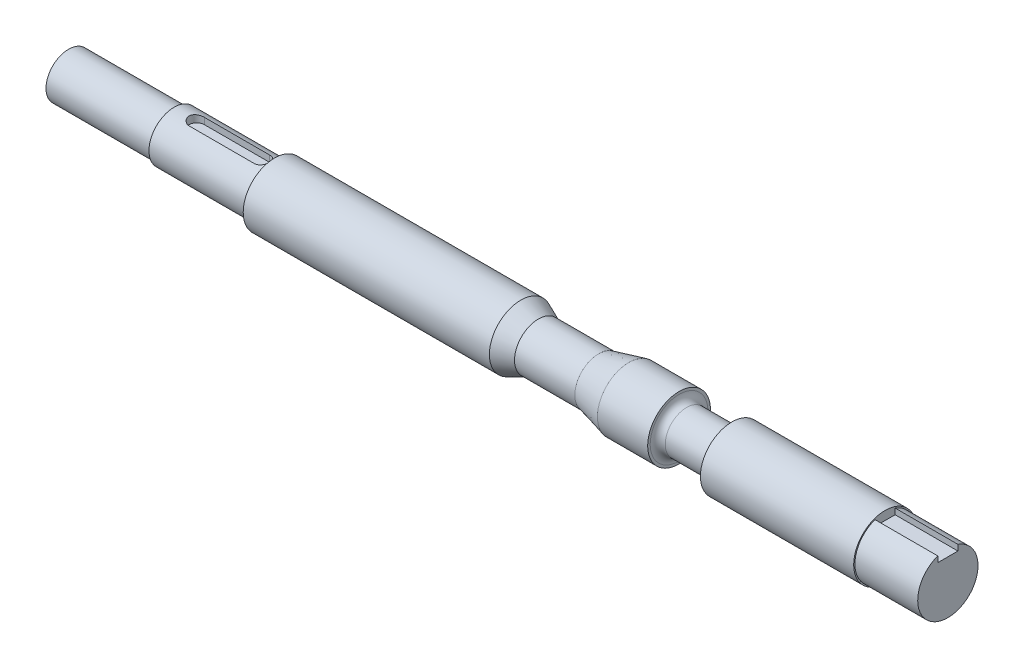
from build123d import *

# Parameters (mm, degrees)
SHOULDER_FILLET_R2_R    = 2
SHOULDER_FILLET_R3_R    = 3
KEYWAY_A_SKETCH_W       = 8
KEYWAY_A_SKETCH_H       = 6
KEYWAY_A_CUT_DEPTH      = 25
KEYWAY_START            = 10
KEYWAY_B_CUT_26X3_DEPTH = 3


with BuildPart() as part:
    # Shaft Profile Sketch → Shaft Body Revolve (revolve)
    with BuildSketch(Plane.XY, mode=Mode.PRIVATE) as shaft_body_revolve_sk:
        Polygon((0, 0), (350, 0), (350, 12), (325, 12), (325, 12.5), (264, 12.5), (264, 8.5), (243, 8.5), (243, 12.5), (223, 12.5), (211, 9.5), (187, 9.5), (180, 12.5), (82, 12.5), (82, 10), (42, 10), (42, 9), (0, 9), align=None)
    revolve(shaft_body_revolve_sk.sketch.rotate(Axis((0, 0, 0), (1, 0, 0)), 90), axis=Axis((0, 0, 0), (1, 0, 0)))

    # Shoulder Fillet R2
    shoulder_fillet_r2_edges = [part.edges().sort_by_distance(p)[0] for p in [
        (264, 0, -8.5),
    ]]
    fillet(shoulder_fillet_r2_edges, radius=SHOULDER_FILLET_R2_R)

    # Shoulder Fillet R3
    shoulder_fillet_r3_edges = [part.edges().sort_by_distance(p)[0] for p in [
        (243, 0, -8.5),
    ]]
    fillet(shoulder_fillet_r3_edges, radius=SHOULDER_FILLET_R3_R)

    # Keyway A Sketch → Keyway A Cut (cut)
    with BuildSketch(Plane(origin=(350, 0, 0), x_dir=(0, 0, -1), z_dir=(1, 0, 0))):
        with Locations((0, 12)):
            Rectangle(KEYWAY_A_SKETCH_W, KEYWAY_A_SKETCH_H)
    extrude(amount=-KEYWAY_A_CUT_DEPTH, mode=Mode.SUBTRACT)

    # Keyway B Sketch 26x3 → Keyway B Cut 26x3 (cut)
    with BuildSketch(Plane(origin=(0, 0, 0), x_dir=(1, 0, 0), z_dir=(0, 1, 0)).offset(KEYWAY_START)):
        with BuildLine():
            Line((51, 3), (77, 3))
            ThreePointArc((77, 3), (80, 0), (77, -3))
            Line((77, -3), (51, -3))
            ThreePointArc((51, -3), (48, 0), (51, 3))
        make_face()
    extrude(amount=-KEYWAY_B_CUT_26X3_DEPTH, mode=Mode.SUBTRACT)


solid = part.part
